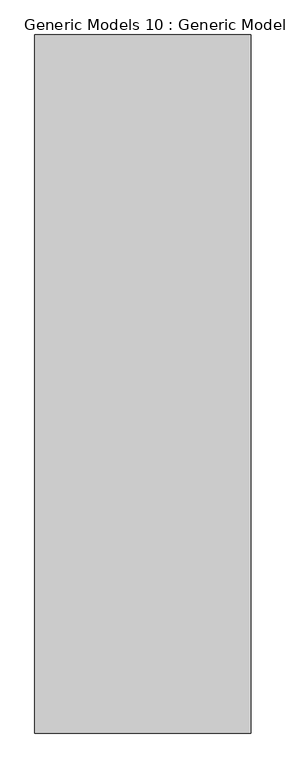
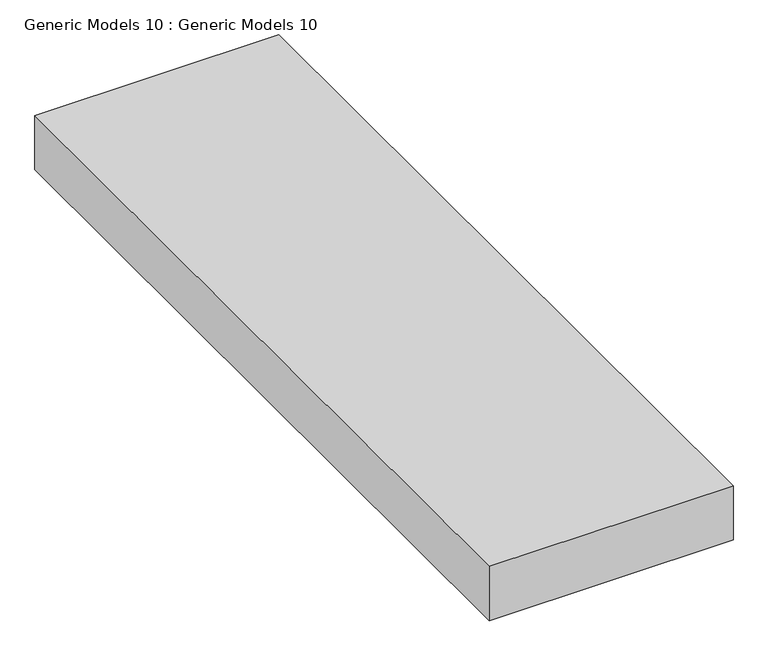
"""IFC4 building model written with IfcOpenShell, lengths in millimetres: proxy geometry, Generic Models 10 : Generic Models 10."""

from ifc_helpers import new_model, si_unit, frame, origin, place, context, project, spatial, polyline, outline, extrude, source, transform, mapped, element, save


def generic_models_10_generic_models_10_282af4fe(model_context):
    return source(origin(), model_context, "Body", "SweptSolid", [
        extrude(outline(polyline([(-22493.3161422, -8877.8914604), (-21845.6161422, -8877.8914604), (-21845.6161422, -10967.2171312), (-22493.3161422, -10967.2171312), (-22493.3161422, -8877.8914604)])), frame((0.0, 0.0, 2454.0538094), z_axis=(0.0, 0.0, 1.0), x_axis=(1.0, 0.0, 0.0)), (0.0, 0.0, 1.0), 152.4),
    ])


if __name__ == "__main__":
    model = new_model("IFC4")
    model_context = context("Model", 3, world=origin())
    ifc_project = project(units=[si_unit("LENGTHUNIT", "METRE", prefix="MILLI")], contexts=[model_context])
    site = spatial("IfcSite", under=ifc_project)
    building = spatial("IfcBuilding", under=site)
    placement = place(None, origin())
    generic_models_10_generic_models_10_shape = generic_models_10_generic_models_10_282af4fe(model_context)
    element("IfcBuildingElementProxy", 1, Name="Generic Models 10 : Generic Models 10", ObjectType="Generic Models 10 : Generic Models 10", at=placement, inside=building, context=model_context, shape_type="MappedRepresentation", body=[
        mapped(generic_models_10_generic_models_10_shape, transform((0.0, 0.0, 0.0), x_axis=(1.0, 0.0, 0.0), y_axis=(0.0, 1.0, 0.0), z_axis=(0.0, 0.0, 1.0))),
    ])
    save(model, "model.ifc")
